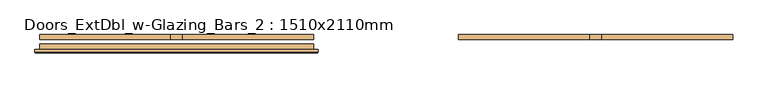
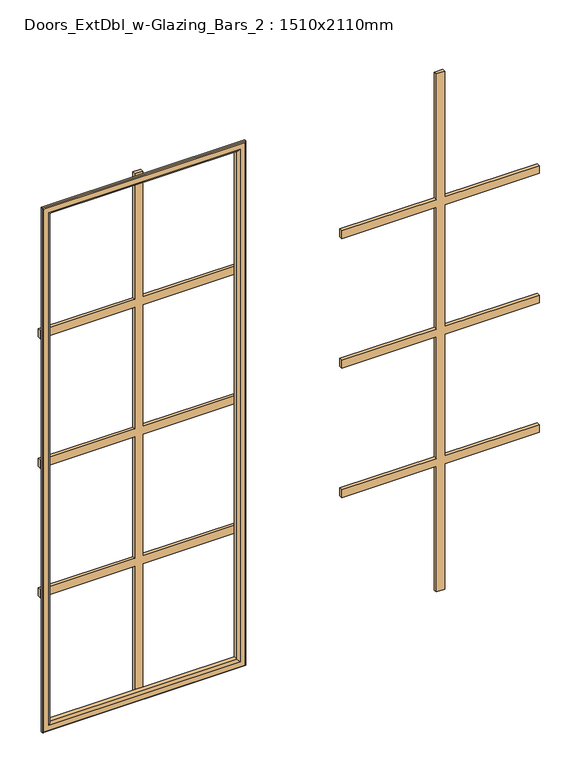
"""IFC4 building model written with IfcOpenShell, lengths in millimetres: door geometry, Doors_ExtDbl_w-Glazing_Bars_2 : 1510x2110mm."""

from ifc_helpers import new_model, si_unit, frame, origin, place, context, project, spatial, polyline, ellipse_curve, outline, extrude, source, transform, mapped, element, save
from ifc_brep_helpers import plane_surface, cylinder_surface, advanced_brep


def doors_extdbl_w_glazing_bars_2_1510x2110mm_b3535315(model_context):
    return source(origin(), model_context, "Body", "SolidModel", [
        advanced_brep(
        [(-611.5, -16.4, 1966.5), (-611.5, -12.4, 1966.5), (-611.5, -12.4, 625.5), (-611.5, -16.4, 625.5), (-609.5, -18.4, 1964.5), (-609.5, -18.4, 627.5), (-591.5, -13.4, 1946.5), (-596.5, -18.4, 1951.5), (-596.5, -18.4, 640.5), (-591.5, -13.4, 645.5), (-591.5, -2.4, 1946.5), (-591.5, -2.4, 645.5), (-603.5, -12.4, 1958.5), (-603.5, -2.4, 1958.5), (-603.5, -2.4, 633.5), (-603.5, -12.4, 633.5), (-118.5, -12.4, 625.5), (-118.5, -16.4, 625.5), (-120.5, -18.4, 627.5), (-133.5, -18.4, 640.5), (-138.5, -13.4, 645.5), (-138.5, -2.4, 645.5), (-126.5, -2.4, 633.5), (-126.5, -12.4, 633.5), (-118.5, -12.4, 1966.5), (-118.5, -16.4, 1966.5), (-120.5, -18.4, 1964.5), (-133.5, -18.4, 1951.5), (-138.5, -13.4, 1946.5), (-138.5, -2.4, 1946.5), (-126.5, -2.4, 1958.5), (-126.5, -12.4, 1958.5)],
        [
            (0, 1),
            (1, 2),
            (2, 3),
            (3, 0),
            (4, 0, ellipse_curve(frame((-609.5, -16.4, 1964.5), z_axis=(-0.707106781186543, 0.0, -0.707106781186552), x_axis=(-0.707106781186552, 0.0, 0.7071067811865429)), 2.8284271, 2.0)),
            (3, 5, ellipse_curve(frame((-609.5, -16.4, 627.5), z_axis=(-0.7071067811865521, 0.0, 0.7071067811865428), x_axis=(0.7071067811865427, 0.0, 0.7071067811865523)), 2.8284271, 2.0)),
            (5, 4),
            (6, 7, ellipse_curve(frame((-596.5, -13.4, 1951.5), z_axis=(-0.707106781186543, 0.0, -0.707106781186552), x_axis=(-0.707106781186552, 0.0, 0.7071067811865429)), 7.0710678, 5.0)),
            (7, 8),
            (8, 9, ellipse_curve(frame((-596.5, -13.4, 640.5), z_axis=(-0.7071067811865521, 0.0, 0.7071067811865428), x_axis=(0.7071067811865427, 0.0, 0.7071067811865523)), 7.0710678, 5.0)),
            (9, 6),
            (10, 6),
            (9, 11),
            (11, 10),
            (12, 13),
            (13, 14),
            (14, 15),
            (15, 12),
            (2, 16),
            (16, 17),
            (17, 3),
            (17, 18, ellipse_curve(frame((-120.5, -16.4, 627.5), z_axis=(-0.7071067811865428, 0.0, -0.7071067811865521), x_axis=(-0.7071067811865522, 0.0, 0.7071067811865427)), 2.8284271, 2.0)),
            (18, 5),
            (8, 19),
            (19, 20, ellipse_curve(frame((-133.5, -13.4, 640.5), z_axis=(-0.7071067811865428, 0.0, -0.7071067811865521), x_axis=(-0.7071067811865522, 0.0, 0.7071067811865427)), 7.0710678, 5.0)),
            (20, 9),
            (20, 21),
            (21, 11),
            (14, 22),
            (22, 23),
            (23, 15),
            (16, 24),
            (24, 25),
            (25, 17),
            (25, 26, ellipse_curve(frame((-120.5, -16.4, 1964.5), z_axis=(0.707106781186552, 0.0, -0.7071067811865429), x_axis=(-0.7071067811865428, 0.0, -0.7071067811865521)), 2.8284271, 2.0)),
            (26, 18),
            (19, 27),
            (27, 28, ellipse_curve(frame((-133.5, -13.4, 1951.5), z_axis=(0.707106781186552, 0.0, -0.7071067811865429), x_axis=(-0.7071067811865428, 0.0, -0.7071067811865521)), 7.0710678, 5.0)),
            (28, 20),
            (28, 29),
            (29, 21),
            (22, 30),
            (30, 31),
            (31, 23),
            (24, 1),
            (0, 25),
            (4, 26),
            (7, 27),
            (6, 28),
            (10, 29),
            (13, 30),
            (12, 31),
        ],
        [
            plane_surface(frame((-611.5, -12.4, 1966.5), z_axis=(-1.0, 0.0, 0.0), x_axis=(0.0, 0.0, -1.0))),
            cylinder_surface(frame((-609.5, -16.4, 1958.5), z_axis=(0.0, 0.0, 1.0), x_axis=(-1.0, 0.0, 0.0)), 2.0),
            cylinder_surface(frame((-596.5, -13.4, 1958.5), z_axis=(0.0, 0.0, 1.0), x_axis=(-1.0, 0.0, 0.0)), 5.0),
            plane_surface(frame((-591.5, -13.4, 1946.5), z_axis=(1.0, 0.0, 0.0), x_axis=(0.0, 0.0, -1.0))),
            plane_surface(frame((-603.5, -2.4, 1958.5), z_axis=(-1.0, 0.0, 0.0), x_axis=(0.0, 0.0, -1.0))),
            plane_surface(frame((-611.5, -12.4, 625.5), z_axis=(0.0, 0.0, -1.0), x_axis=(1.0, 0.0, 0.0))),
            cylinder_surface(frame((-603.5, -16.4, 627.5), z_axis=(-1.0, 0.0, 0.0), x_axis=(0.0, 0.0, -1.0)), 2.0),
            cylinder_surface(frame((-603.5, -13.4, 640.5), z_axis=(-1.0, 0.0, 0.0), x_axis=(0.0, 0.0, -1.0)), 5.0),
            plane_surface(frame((-591.5, -13.4, 645.5), z_axis=(0.0, 0.0, 1.0), x_axis=(1.0, 0.0, 0.0))),
            plane_surface(frame((-603.5, -2.4, 633.5), z_axis=(0.0, 0.0, -1.0), x_axis=(1.0, 0.0, 0.0))),
            plane_surface(frame((-118.5, -12.4, 625.5), z_axis=(1.0, 0.0, 0.0), x_axis=(0.0, 0.0, 1.0))),
            cylinder_surface(frame((-120.5, -16.4, 633.5), z_axis=(0.0, 0.0, -1.0), x_axis=(1.0, 0.0, 0.0)), 2.0),
            cylinder_surface(frame((-133.5, -13.4, 633.5), z_axis=(0.0, 0.0, -1.0), x_axis=(1.0, 0.0, 0.0)), 5.0),
            plane_surface(frame((-138.5, -13.4, 645.5), z_axis=(-1.0, 0.0, 0.0), x_axis=(0.0, 0.0, 1.0))),
            plane_surface(frame((-126.5, -2.4, 633.5), z_axis=(1.0, 0.0, 0.0), x_axis=(0.0, 0.0, 1.0))),
            plane_surface(frame((-118.5, -12.4, 1966.5), z_axis=(0.0, 0.0, 1.0), x_axis=(-1.0, 0.0, 0.0))),
            cylinder_surface(frame((-126.5, -16.4, 1964.5), z_axis=(1.0, 0.0, 0.0), x_axis=(0.0, 0.0, 1.0)), 2.0),
            plane_surface(frame((-120.5, -18.4, 1964.5), z_axis=(0.0, -1.0, 0.0), x_axis=(-1.0, 0.0, 0.0))),
            cylinder_surface(frame((-126.5, -13.4, 1951.5), z_axis=(1.0, 0.0, 0.0), x_axis=(0.0, 0.0, 1.0)), 5.0),
            plane_surface(frame((-138.5, -13.4, 1946.5), z_axis=(0.0, 0.0, -1.0), x_axis=(-1.0, 0.0, 0.0))),
            plane_surface(frame((-138.5, -2.4, 1946.5), z_axis=(0.0, 1.0, 0.0), x_axis=(-1.0, 0.0, 0.0))),
            plane_surface(frame((-126.5, -2.4, 1958.5), z_axis=(0.0, 0.0, 1.0), x_axis=(-1.0, 0.0, 0.0))),
            plane_surface(frame((-126.5, -12.4, 1958.5), z_axis=(0.0, 1.0, 0.0), x_axis=(-1.0, 0.0, 0.0))),
        ],
        [
            (0, [[1, 2, 3, 4]]),
            (1, [[5, -4, 6, 7]]),
            (2, [[8, 9, 10, 11]]),
            (3, [[12, -11, 13, 14]]),
            (4, [[15, 16, 17, 18]]),
            (5, [[-3, 19, 20, 21]]),
            (6, [[-6, -21, 22, 23]]),
            (7, [[-10, 24, 25, 26]]),
            (8, [[-13, -26, 27, 28]]),
            (9, [[-17, 29, 30, 31]]),
            (10, [[-20, 32, 33, 34]]),
            (11, [[-22, -34, 35, 36]]),
            (12, [[-25, 37, 38, 39]]),
            (13, [[-27, -39, 40, 41]]),
            (14, [[-30, 42, 43, 44]]),
            (15, [[-33, 45, -1, 46]]),
            (16, [[-35, -46, -5, 47]]),
            (17, [[-23, -36, -47, -7], [48, -37, -24, -9]]),
            (18, [[-38, -48, -8, 49]]),
            (19, [[-40, -49, -12, 50]]),
            (20, [[51, -42, -29, -16], [-28, -41, -50, -14]]),
            (21, [[-43, -51, -15, 52]]),
            (22, [[-45, -32, -19, -2], [-31, -44, -52, -18]]),
        ],
    ),
        extrude(outline(polyline([(1637.25, -355.0), (1958.5, -355.0), (1958.5, -375.0), (1637.25, -375.0), (1637.25, -603.5), (1617.25, -603.5), (1617.25, -375.0), (1306.0, -375.0), (1306.0, -603.5), (1286.0, -603.5), (1286.0, -375.0), (974.75, -375.0), (974.75, -603.5), (954.75, -603.5), (954.75, -375.0), (633.5, -375.0), (633.5, -355.0), (954.75, -355.0), (954.75, -126.5), (974.75, -126.5), (974.75, -355.0), (1286.0, -355.0), (1286.0, -126.5), (1306.0, -126.5), (1306.0, -355.0), (1617.25, -355.0), (1617.25, -126.5), (1637.25, -126.5), (1637.25, -355.0)])), frame((0.0, 5.6, 0.0), z_axis=(0.0, 1.0, 0.0), x_axis=(0.0, 0.0, 1.0)), (0.0, 0.0, 1.0), 8.0),
        extrude(outline(polyline([(1637.25, 375.0), (1958.5, 375.0), (1958.5, 355.0), (1637.25, 355.0), (1637.25, 126.5), (1617.25, 126.5), (1617.25, 355.0), (1306.0, 355.0), (1306.0, 126.5), (1286.0, 126.5), (1286.0, 355.0), (974.75, 355.0), (974.75, 126.5), (954.75, 126.5), (954.75, 355.0), (633.5, 355.0), (633.5, 375.0), (954.75, 375.0), (954.75, 603.5), (974.75, 603.5), (974.75, 375.0), (1286.0, 375.0), (1286.0, 603.5), (1306.0, 603.5), (1306.0, 375.0), (1617.25, 375.0), (1617.25, 603.5), (1637.25, 603.5), (1637.25, 375.0)])), frame((0.0, 5.6, 0.0), z_axis=(0.0, 1.0, 0.0), x_axis=(0.0, 0.0, 1.0)), (0.0, 0.0, 1.0), 8.0),
    ])


if __name__ == "__main__":
    model = new_model("IFC4")
    model_context = context("Model", 3, world=origin())
    ifc_project = project(units=[si_unit("LENGTHUNIT", "METRE", prefix="MILLI")], contexts=[model_context])
    site = spatial("IfcSite", under=ifc_project)
    building = spatial("IfcBuilding", under=site)
    placement = place(None, origin())
    doors_extdbl_w_glazing_bars_2_1510x2110mm_shape = doors_extdbl_w_glazing_bars_2_1510x2110mm_b3535315(model_context)
    element("IfcDoor", 1, ObjectType="Doors_ExtDbl_w-Glazing_Bars_2 : 1510x2110mm", at=placement, inside=building, context=model_context, shape_type="MappedRepresentation", body=[
        mapped(doors_extdbl_w_glazing_bars_2_1510x2110mm_shape, transform((0.0, 0.0, 0.0), x_axis=(1.0, 0.0, 0.0), y_axis=(0.0, 1.0, 0.0), z_axis=(0.0, 0.0, 1.0))),
    ])
    save(model, "model.ifc")

# Revit data of these elements
# Type "Doors_ExtDbl_w-Glazing_Bars_2 : 1510x2110mm"
#   Type Mark = "15"
#   Type Comments = "External Double"
#   Operation = "DoubleDoorSingleSwing"
#   Construction Type Id = "GSP4R"
#   Keynote = "L20"
#   Analytic Construction = "1/8 in Pilkington single glazing"
#   Wrap Layers (Int) from Ext = 0' - 6.98819"
#   Wrap Layers (Ext) from Ext = 0' - 4.03543"
#   Visual Light Transmittance = 0.9
#   Top of Intermediate Rail = 1' - 10.6378"
#   Thickness = 0' - 1.73228"
#   Stile Shutting = 0' - 4.92126"
#   Stile - Top Rail = 0' - 3.93701"
#   Stile - Lock Rail = 0' - 3.93701"
#   Stile - Hanging = 0' - 3.93701"
#   Stile - Bottom Rail = 0' - 6.88976"
#   Solar Heat Gain Coefficient = 0.78
#   Rough Width = 4' - 11.44882"
#   Rough Height = 6' - 11.07087"
#   O/A Frame Width = 0' - 2.51969"
#   Heat Transfer Coefficient (U) = 0.6496 BTU/(h·ft²·°F)
#   Handle Z Distance = 3' - 5.33858"
#   Glazing Thickness = 0' - 0.94488"
#   Glazing Bar Thickness = 0' - 0.7874"
#   FrameWidth = 0' - 1.65354"
#   FrameOffset - External = 0' - 0.98425"
#   FrameDepth = 0' - 3.50394"
#   Door Panel Width = 2' - 3.6378"
#   Door Panel Thickness = 0' - 1.73228"
#   Door Panel Height = 6' - 6.74016"
#   Cill Thickness = 0' - 2.14567"
#   Cill Projection = 0' - 1.1811"
#   Handle X Distance = 0' - 2.95276"
#   Height = 6' - 11.07087"
#   Structural Tolerance = 0' - 0.25591"
#   Tolerance = 0' - 0.11811"
#   Undercut = 0' - 0.15748"
#   Width = 4' - 11.44882"
#   Cill Extension = 0' - 0.98425"
#   Cavity Closer Width = 0' - 1.9685"
#   Cavity Closer Offset from Ext = 0' - 4.03543"
#   Cavity Closer Depth = 0' - 3.34646"
#   Vis - Ironmongery = yes
#   Vis - Glazing Bars = yes
#   Vis - Cavity Closers = yes
#   Define Thermal Properties by = 1
#   Function = 1
#   Material Glazing Bars = Door - Panel
#   Material Glass = Door - Glazing
#   Material Door = Door - Panel
#   Material Frame = Door - Frame/Mullion
#   Material Ironmongery = Door - Handle
#   Wall Closure = (empty or 0)
#   Assembly Code = ""
# Element 1 (IfcDoor, "Doors_ExtDbl_w-Glazing_Bars_2 : 1510x2110mm")
#   Materials on its faces: "Door - Panel", "Door - Handle", "Door - Frame/Mullion", "Door - Glazing"
# Materials
#   "Door - Panel": class "Wood", colour RGB 210 159 95, transparency 0, Cost = 0
#   "Door - Glazing": colour RGB 0 0 255, transparency 0.75
#   "Door - Frame/Mullion": class "Wood", colour RGB 212 179 113, transparency 0
#   "Door - Handle": colour RGB 247 247 247, transparency 0
